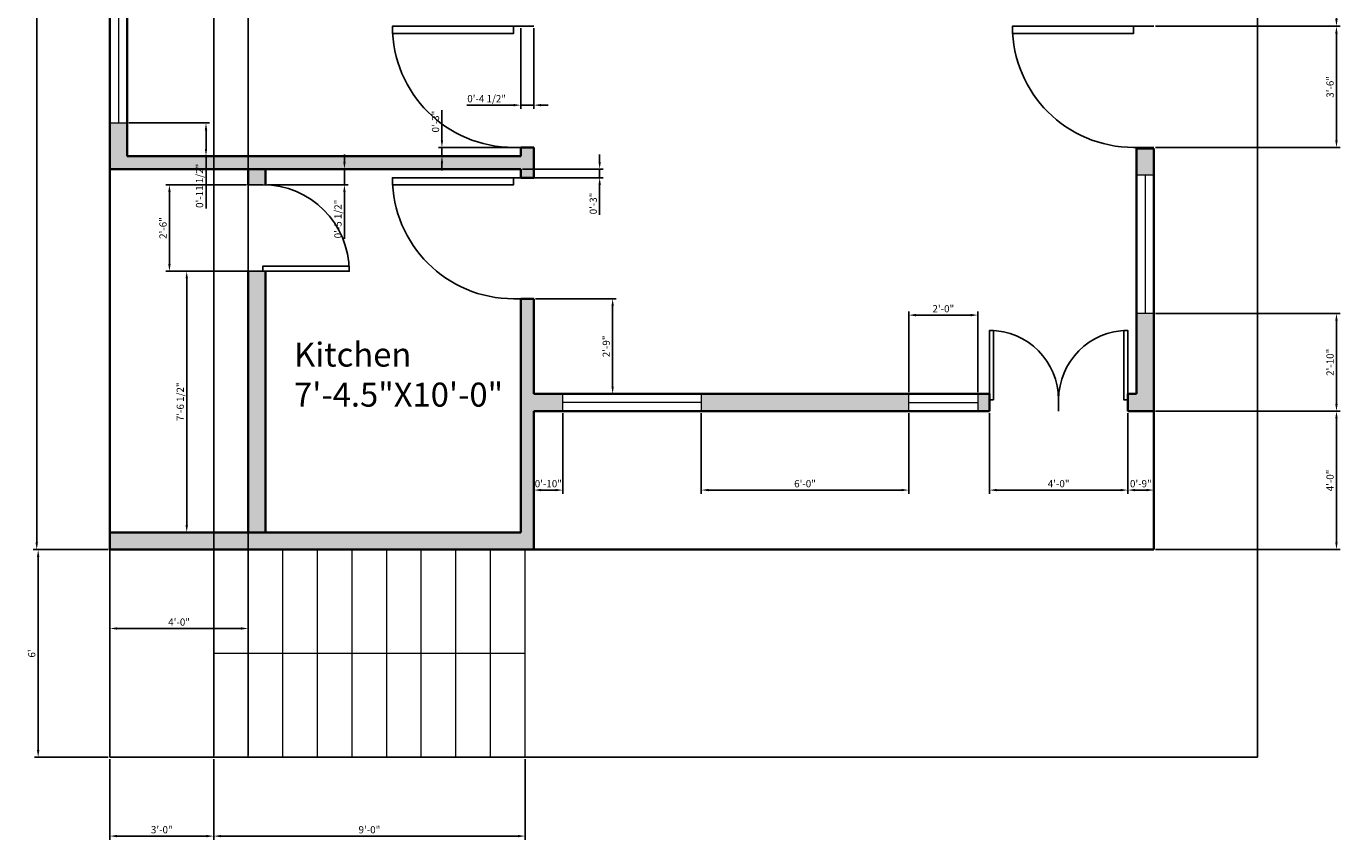
# Model space of a CAD drawing. Units: inches. Extents: x 1129603 to 1130059, y 1058961 to 1059552.
# Tile 1 of 2: x 1129603 to 1130059, y 1058961 to 1059243. Entities that reach past the tile are written whole.
import ezdxf

# ---------------------------------------------------------------- set-up
doc = ezdxf.new("R2010")
doc.units = ezdxf.units.IN
for name, color, linetype, lineweight in [('A-ANNO-DIMS', 2, 'Continuous', 18), ('A-AREA-IDEN', 7, 'Continuous', 25), ('A-DOOR', 3, 'Continuous', 25), ('A-FLOR-STRS', 7, 'Continuous', 18), ('A-GLAZ', 4, 'Continuous', 18), ('A-WALL-PATT', 9, 'Continuous', 13), ('C-PROP', 8, 'Continuous', 25), ('walls', 7, 'Continuous', 35)]:
    doc.layers.add(name, color=color, linetype=linetype, lineweight=lineweight)
doc.styles.get("Standard").update_dxf_attribs({"font": 'arial.ttf'})
doc.dimstyles.new('ISO-25', dxfattribs={"dimtxt": 2.5, "dimasz": 2.5, "dimexe": 1.25, "dimexo": 0.625, "dimtad": 1, "dimlunit": 4, "dimtxsty": 'Standard', "dimcen": 2.5, "dimadec": 0, "dimazin": 0, "dimtfac": 1, "dimtmove": 0, "dimatfit": 3, "dimfxl": 1, "dimarcsym": 0})

# ---------------------------------------------------------------- blocks, each defined once
blk = doc.blocks.new('*U2')
for p, q in [((0, 0), (0, -5)), ((30, 0), (30, -5))]:
    blk.add_line(p, q)
blk.add_lwpolyline([(0, 0), (0, 30), (1.75, 30), (1.75, 0)], close=True)
blk.add_arc((0, 0), 30, 0, 90)
blk = doc.blocks.new('*D5')
at = {"layer": 'A-ANNO-DIMS', "color": 0, "lineweight": -2, "transparency": 16777216}
for p, q in [((1129630.99, 1059520.87), (1129605, 1059520.87)), ((1129606.25, 1059518.37), (1129606.25, 1059064.37)), ((1129630.99, 1059061.87), (1129605, 1059061.87))]:
    blk.add_line(p, q, dxfattribs=at)
at = {"layer": 'A-ANNO-DIMS', "color": 0, "transparency": 16777216}
for points in [[(1129605.83, 1059518.37), (1129606.66, 1059518.37), (1129606.25, 1059520.87)], [(1129605.83, 1059064.37), (1129606.66, 1059064.37), (1129606.25, 1059061.87)]]:
    blk.add_solid(points, dxfattribs=at)
at = {"layer": 'Defpoints', "color": 0, "transparency": 16777216}
for p in [(1129631.62, 1059520.87), (1129606.25, 1059061.87), (1129631.62, 1059061.87)]:
    blk.add_point(p, dxfattribs=at)
at = {"layer": 'A-ANNO-DIMS', "color": 0, "transparency": 16777216, "insert": (1129604.34, 1059291.37), "char_height": 2.5, "attachment_point": 5, "rotation": 90}
blk.add_mtext('38\'-3"', dxfattribs=at)
blk = doc.blocks.new('*D6')
at = {"layer": 'A-ANNO-DIMS', "color": 0, "lineweight": -2, "transparency": 16777216}
for p, q in [((1129630.99, 1059061.87), (1129605.51, 1059061.87)), ((1129606.76, 1059059.37), (1129606.76, 1058992.37)), ((1129630.99, 1058989.87), (1129605.51, 1058989.87))]:
    blk.add_line(p, q, dxfattribs=at)
at = {"layer": 'A-ANNO-DIMS', "color": 0, "transparency": 16777216}
for points in [[(1129606.34, 1059059.37), (1129607.17, 1059059.37), (1129606.76, 1059061.87)], [(1129606.34, 1058992.37), (1129607.17, 1058992.37), (1129606.76, 1058989.87)]]:
    blk.add_solid(points, dxfattribs=at)
at = {"layer": 'Defpoints', "color": 0, "transparency": 16777216}
for p in [(1129631.62, 1059061.87), (1129606.76, 1058989.87), (1129631.62, 1058989.87)]:
    blk.add_point(p, dxfattribs=at)
at = {"layer": 'A-ANNO-DIMS', "color": 0, "transparency": 16777216, "insert": (1129604.85, 1059025.87), "char_height": 2.5, "attachment_point": 5, "rotation": 90}
blk.add_mtext("6'", dxfattribs=at)
blk = doc.blocks.new('WIN-48IN')
for p, q in [((0, 6), (48, 6)), ((0, 0), (0, 6)), ((48, 6), (48, 0)), ((0, 3), (48, 3)), ((48, 0), (0, 0))]:
    blk.add_line(p, q)
blk = doc.blocks.new('*D13')
at = {"layer": 'A-ANNO-DIMS', "color": 0, "lineweight": -2, "transparency": 16777216}
for p, q in [((1129638.24, 1059209.84), (1129666.21, 1059209.84)), ((1129664.96, 1059207.34), (1129664.96, 1059200.87)), ((1129638.24, 1059198.37), (1129666.21, 1059198.37)), ((1129664.96, 1059198.37), (1129664.96, 1059180.21))]:
    blk.add_line(p, q, dxfattribs=at)
at = {"layer": 'A-ANNO-DIMS', "color": 0, "transparency": 16777216}
for points in [[(1129664.54, 1059207.34), (1129665.37, 1059207.34), (1129664.96, 1059209.84)], [(1129664.54, 1059200.87), (1129665.37, 1059200.87), (1129664.96, 1059198.37)]]:
    blk.add_solid(points, dxfattribs=at)
at = {"layer": 'Defpoints', "color": 0, "transparency": 16777216}
for p in [(1129637.62, 1059209.84), (1129637.62, 1059198.37), (1129664.96, 1059198.37)]:
    blk.add_point(p, dxfattribs=at)
at = {"layer": 'A-ANNO-DIMS', "color": 0, "transparency": 16777216, "insert": (1129663.04, 1059188.04), "char_height": 2.5, "attachment_point": 5, "rotation": 90}
blk.add_mtext('0\'-11 1/2"', dxfattribs=at)
blk = doc.blocks.new('*D16')
at = {"layer": 'A-ANNO-DIMS', "color": 0, "lineweight": -2, "transparency": 16777216}
for p, q in [((1129994.24, 1059288.97), (1130058.21, 1059288.97)), ((1130056.96, 1059245.87), (1130056.96, 1059286.47)), ((1129994.24, 1059243.37), (1130058.21, 1059243.37))]:
    blk.add_line(p, q, dxfattribs=at)
at = {"layer": 'A-ANNO-DIMS', "color": 0, "transparency": 16777216}
for points in [[(1130056.54, 1059286.47), (1130057.37, 1059286.47), (1130056.96, 1059288.97)], [(1130056.54, 1059245.87), (1130057.37, 1059245.87), (1130056.96, 1059243.37)]]:
    blk.add_solid(points, dxfattribs=at)
at = {"layer": 'Defpoints', "color": 0, "transparency": 16777216}
for p in [(1129993.62, 1059288.97), (1130056.96, 1059288.97), (1129993.62, 1059243.37)]:
    blk.add_point(p, dxfattribs=at)
at = {"layer": 'A-ANNO-DIMS', "color": 0, "transparency": 16777216, "insert": (1130055.04, 1059266.17), "char_height": 2.5, "attachment_point": 5, "rotation": 90}
blk.add_mtext('3\'-9 1/2"', dxfattribs=at)
blk = doc.blocks.new('*D17')
at = {"layer": 'A-ANNO-DIMS', "color": 0, "lineweight": -2, "transparency": 16777216}
for p, q in [((1129994.24, 1059243.37), (1130058.21, 1059243.37)), ((1130056.96, 1059203.87), (1130056.96, 1059240.87)), ((1129994.24, 1059201.37), (1130058.21, 1059201.37))]:
    blk.add_line(p, q, dxfattribs=at)
at = {"layer": 'A-ANNO-DIMS', "color": 0, "transparency": 16777216}
for points in [[(1130056.54, 1059240.87), (1130057.37, 1059240.87), (1130056.96, 1059243.37)], [(1130056.54, 1059203.87), (1130057.37, 1059203.87), (1130056.96, 1059201.37)]]:
    blk.add_solid(points, dxfattribs=at)
at = {"layer": 'Defpoints', "color": 0, "transparency": 16777216}
for p in [(1129993.62, 1059243.37), (1130056.96, 1059243.37), (1129993.62, 1059201.37)]:
    blk.add_point(p, dxfattribs=at)
at = {"layer": 'A-ANNO-DIMS', "color": 0, "transparency": 16777216, "insert": (1130055.06, 1059222.37), "char_height": 2.5, "attachment_point": 5, "rotation": 90}
blk.add_mtext('3\'-6"', dxfattribs=at)
blk = doc.blocks.new('*D18')
at = {"layer": 'A-ANNO-DIMS', "color": 0, "lineweight": -2, "transparency": 16777216}
for p, q in [((1129994.24, 1059143.81), (1130058.21, 1059143.81)), ((1130056.96, 1059112.37), (1130056.96, 1059141.31)), ((1129994.24, 1059109.87), (1130058.21, 1059109.87))]:
    blk.add_line(p, q, dxfattribs=at)
at = {"layer": 'A-ANNO-DIMS', "color": 0, "transparency": 16777216}
for points in [[(1130056.54, 1059141.31), (1130057.37, 1059141.31), (1130056.96, 1059143.81)], [(1130056.54, 1059112.37), (1130057.37, 1059112.37), (1130056.96, 1059109.87)]]:
    blk.add_solid(points, dxfattribs=at)
at = {"layer": 'Defpoints', "color": 0, "transparency": 16777216}
for p in [(1129993.62, 1059143.81), (1130056.96, 1059143.81), (1129993.62, 1059109.87)]:
    blk.add_point(p, dxfattribs=at)
at = {"layer": 'A-ANNO-DIMS', "color": 0, "transparency": 16777216, "insert": (1130055.06, 1059126.84), "char_height": 2.5, "attachment_point": 5, "rotation": 90}
blk.add_mtext('2\'-10"', dxfattribs=at)
blk = doc.blocks.new('*D19')
at = {"layer": 'A-ANNO-DIMS', "color": 0, "lineweight": -2, "transparency": 16777216}
for p, q in [((1129994.24, 1059109.87), (1130058.21, 1059109.87)), ((1130056.96, 1059107.37), (1130056.96, 1059064.37)), ((1129994.24, 1059061.87), (1130058.21, 1059061.87))]:
    blk.add_line(p, q, dxfattribs=at)
at = {"layer": 'A-ANNO-DIMS', "color": 0, "transparency": 16777216}
for points in [[(1130056.54, 1059107.37), (1130057.37, 1059107.37), (1130056.96, 1059109.87)], [(1130056.54, 1059064.37), (1130057.37, 1059064.37), (1130056.96, 1059061.87)]]:
    blk.add_solid(points, dxfattribs=at)
at = {"layer": 'Defpoints', "color": 0, "transparency": 16777216}
for p in [(1129993.62, 1059109.87), (1129993.62, 1059061.87), (1130056.96, 1059061.87)]:
    blk.add_point(p, dxfattribs=at)
at = {"layer": 'A-ANNO-DIMS', "color": 0, "transparency": 16777216, "insert": (1130055.06, 1059085.87), "char_height": 2.5, "attachment_point": 5, "rotation": 90}
blk.add_mtext('4\'-0"', dxfattribs=at)
blk = doc.blocks.new('*D20')
at = {"layer": 'A-ANNO-DIMS', "color": 0, "lineweight": -2, "transparency": 16777216}
for p, q in [((1129631.62, 1059061.25), (1129631.62, 1059033.28)), ((1129679.62, 1059061.25), (1129679.62, 1059033.28)), ((1129677.12, 1059034.53), (1129634.12, 1059034.53))]:
    blk.add_line(p, q, dxfattribs=at)
at = {"layer": 'A-ANNO-DIMS', "color": 0, "transparency": 16777216}
for points in [[(1129634.12, 1059034.95), (1129634.12, 1059034.12), (1129631.62, 1059034.53)], [(1129677.12, 1059034.95), (1129677.12, 1059034.12), (1129679.62, 1059034.53)]]:
    blk.add_solid(points, dxfattribs=at)
at = {"layer": 'Defpoints', "color": 0, "transparency": 16777216}
for p in [(1129631.62, 1059061.87), (1129679.62, 1059061.87), (1129631.62, 1059034.53)]:
    blk.add_point(p, dxfattribs=at)
at = {"layer": 'A-ANNO-DIMS', "color": 0, "transparency": 16777216, "insert": (1129655.62, 1059036.43), "char_height": 2.5, "attachment_point": 5}
blk.add_mtext('4\'-0"', dxfattribs=at)
blk = doc.blocks.new('*D21')
at = {"layer": 'A-ANNO-DIMS', "color": 0, "lineweight": -2, "transparency": 16777216}
for p, q in [((1129631.62, 1058989.25), (1129631.62, 1058961.28)), ((1129667.62, 1058989.25), (1129667.62, 1058961.28)), ((1129634.12, 1058962.53), (1129665.12, 1058962.53))]:
    blk.add_line(p, q, dxfattribs=at)
at = {"layer": 'A-ANNO-DIMS', "color": 0, "transparency": 16777216}
for points in [[(1129634.12, 1058962.95), (1129634.12, 1058962.12), (1129631.62, 1058962.53)], [(1129665.12, 1058962.95), (1129665.12, 1058962.12), (1129667.62, 1058962.53)]]:
    blk.add_solid(points, dxfattribs=at)
at = {"layer": 'Defpoints', "color": 0, "transparency": 16777216}
for p in [(1129631.62, 1058989.87), (1129667.62, 1058989.87), (1129667.62, 1058962.53)]:
    blk.add_point(p, dxfattribs=at)
at = {"layer": 'A-ANNO-DIMS', "color": 0, "transparency": 16777216, "insert": (1129649.62, 1058964.43), "char_height": 2.5, "attachment_point": 5}
blk.add_mtext('3\'-0"', dxfattribs=at)
blk = doc.blocks.new('*D22')
at = {"layer": 'A-ANNO-DIMS', "color": 0, "lineweight": -2, "transparency": 16777216}
for p, q in [((1129667.62, 1058989.25), (1129667.62, 1058961.28)), ((1129775.62, 1058989.25), (1129775.62, 1058961.28)), ((1129670.12, 1058962.53), (1129773.12, 1058962.53))]:
    blk.add_line(p, q, dxfattribs=at)
at = {"layer": 'A-ANNO-DIMS', "color": 0, "transparency": 16777216}
for points in [[(1129670.12, 1058962.95), (1129670.12, 1058962.12), (1129667.62, 1058962.53)], [(1129773.12, 1058962.95), (1129773.12, 1058962.12), (1129775.62, 1058962.53)]]:
    blk.add_solid(points, dxfattribs=at)
at = {"layer": 'Defpoints', "color": 0, "transparency": 16777216}
for p in [(1129667.62, 1058989.87), (1129775.62, 1058989.87), (1129775.62, 1058962.53)]:
    blk.add_point(p, dxfattribs=at)
at = {"layer": 'A-ANNO-DIMS', "color": 0, "transparency": 16777216, "insert": (1129721.62, 1058964.43), "char_height": 2.5, "attachment_point": 5}
blk.add_mtext('9\'-0"', dxfattribs=at)
blk = doc.blocks.new('*D23')
at = {"layer": 'A-ANNO-DIMS', "color": 0, "lineweight": -2, "transparency": 16777216}
for p, q in [((1129667.62, 1058990.5), (1129667.62, 1059549.47)), ((1129670.12, 1059548.22), (1129677.12, 1059548.22)), ((1129679.62, 1058990.5), (1129679.62, 1059549.47))]:
    blk.add_line(p, q, dxfattribs=at)
at = {"layer": 'A-ANNO-DIMS', "color": 0, "transparency": 16777216}
for points in [[(1129670.12, 1059548.63), (1129670.12, 1059547.8), (1129667.62, 1059548.22)], [(1129677.12, 1059548.63), (1129677.12, 1059547.8), (1129679.62, 1059548.22)]]:
    blk.add_solid(points, dxfattribs=at)
at = {"layer": 'Defpoints', "color": 0, "transparency": 16777216}
for p in [(1129679.62, 1059548.22), (1129667.62, 1058989.87), (1129679.62, 1058989.87)]:
    blk.add_point(p, dxfattribs=at)
at = {"layer": 'A-ANNO-DIMS', "color": 0, "transparency": 16777216, "insert": (1129673.62, 1059550.12), "char_height": 2.5, "attachment_point": 5}
blk.add_mtext('1\'-0"', dxfattribs=at)
blk = doc.blocks.new('*D24')
at = {"layer": 'A-ANNO-DIMS', "color": 0, "lineweight": -2, "transparency": 16777216}
for p, q in [((1129936.62, 1059109.25), (1129936.62, 1059081.28)), ((1129984.62, 1059109.25), (1129984.62, 1059081.28)), ((1129982.12, 1059082.53), (1129939.12, 1059082.53))]:
    blk.add_line(p, q, dxfattribs=at)
at = {"layer": 'A-ANNO-DIMS', "color": 0, "transparency": 16777216}
for points in [[(1129939.12, 1059082.95), (1129939.12, 1059082.12), (1129936.62, 1059082.53)], [(1129982.12, 1059082.95), (1129982.12, 1059082.12), (1129984.62, 1059082.53)]]:
    blk.add_solid(points, dxfattribs=at)
at = {"layer": 'Defpoints', "color": 0, "transparency": 16777216}
for p in [(1129936.62, 1059109.87), (1129984.62, 1059109.87), (1129936.62, 1059082.53)]:
    blk.add_point(p, dxfattribs=at)
at = {"layer": 'A-ANNO-DIMS', "color": 0, "transparency": 16777216, "insert": (1129960.62, 1059084.43), "char_height": 2.5, "attachment_point": 5, "rotation": 0}
blk.add_mtext('4\'-0"', dxfattribs=at)
blk = doc.blocks.new('*D25')
at = {"layer": 'A-ANNO-DIMS', "color": 0, "lineweight": -2, "transparency": 16777216}
for p, q in [((1129908.63, 1059116.5), (1129908.63, 1059144.47)), ((1129932.63, 1059116.5), (1129932.63, 1059144.47)), ((1129911.13, 1059143.22), (1129930.13, 1059143.22))]:
    blk.add_line(p, q, dxfattribs=at)
at = {"layer": 'A-ANNO-DIMS', "color": 0, "transparency": 16777216}
for points in [[(1129911.13, 1059143.63), (1129911.13, 1059142.8), (1129908.63, 1059143.22)], [(1129930.13, 1059143.63), (1129930.13, 1059142.8), (1129932.63, 1059143.22)]]:
    blk.add_solid(points, dxfattribs=at)
at = {"layer": 'Defpoints', "color": 0, "transparency": 16777216}
for p in [(1129932.63, 1059143.22), (1129908.63, 1059115.87), (1129932.63, 1059115.87)]:
    blk.add_point(p, dxfattribs=at)
at = {"layer": 'A-ANNO-DIMS', "color": 0, "transparency": 16777216, "insert": (1129920.63, 1059145.12), "char_height": 2.5, "attachment_point": 5}
blk.add_mtext('2\'-0"', dxfattribs=at)
blk = doc.blocks.new('*D26')
at = {"layer": 'A-ANNO-DIMS', "color": 0, "lineweight": -2, "transparency": 16777216}
for p, q in [((1129778.62, 1059109.25), (1129778.62, 1059081.28)), ((1129788.71, 1059109.25), (1129788.71, 1059081.28)), ((1129786.21, 1059082.53), (1129781.12, 1059082.53))]:
    blk.add_line(p, q, dxfattribs=at)
at = {"layer": 'A-ANNO-DIMS', "color": 0, "transparency": 16777216}
for points in [[(1129781.12, 1059082.95), (1129781.12, 1059082.12), (1129778.62, 1059082.53)], [(1129786.21, 1059082.95), (1129786.21, 1059082.12), (1129788.71, 1059082.53)]]:
    blk.add_solid(points, dxfattribs=at)
at = {"layer": 'Defpoints', "color": 0, "transparency": 16777216}
for p in [(1129778.62, 1059109.87), (1129788.71, 1059109.87), (1129778.62, 1059082.53)]:
    blk.add_point(p, dxfattribs=at)
at = {"layer": 'A-ANNO-DIMS', "color": 0, "transparency": 16777216, "insert": (1129783.66, 1059084.43), "char_height": 2.5, "attachment_point": 5, "rotation": 0}
blk.add_mtext('0\'-10"', dxfattribs=at)
blk = doc.blocks.new('*D27')
at = {"layer": 'A-ANNO-DIMS', "color": 0, "lineweight": -2, "transparency": 16777216}
for p, q in [((1129836.71, 1059109.25), (1129836.71, 1059081.28)), ((1129908.63, 1059109.25), (1129908.63, 1059081.28)), ((1129906.13, 1059082.53), (1129839.21, 1059082.53))]:
    blk.add_line(p, q, dxfattribs=at)
at = {"layer": 'A-ANNO-DIMS', "color": 0, "transparency": 16777216}
for points in [[(1129839.21, 1059082.95), (1129839.21, 1059082.12), (1129836.71, 1059082.53)], [(1129906.13, 1059082.95), (1129906.13, 1059082.12), (1129908.63, 1059082.53)]]:
    blk.add_solid(points, dxfattribs=at)
at = {"layer": 'Defpoints', "color": 0, "transparency": 16777216}
for p in [(1129836.71, 1059109.87), (1129908.63, 1059109.87), (1129836.71, 1059082.53)]:
    blk.add_point(p, dxfattribs=at)
at = {"layer": 'A-ANNO-DIMS', "color": 0, "transparency": 16777216, "insert": (1129872.67, 1059084.43), "char_height": 2.5, "attachment_point": 5, "rotation": 0}
blk.add_mtext('6\'-0"', dxfattribs=at)
blk = doc.blocks.new('*D28')
at = {"layer": 'A-ANNO-DIMS', "color": 0, "lineweight": -2, "transparency": 16777216}
for p, q in [((1129984.62, 1059109.25), (1129984.62, 1059081.28)), ((1129993.62, 1059109.25), (1129993.62, 1059081.28)), ((1129991.12, 1059082.53), (1129987.12, 1059082.53))]:
    blk.add_line(p, q, dxfattribs=at)
at = {"layer": 'A-ANNO-DIMS', "color": 0, "transparency": 16777216}
for points in [[(1129987.12, 1059082.95), (1129987.12, 1059082.12), (1129984.62, 1059082.53)], [(1129991.12, 1059082.95), (1129991.12, 1059082.12), (1129993.62, 1059082.53)]]:
    blk.add_solid(points, dxfattribs=at)
at = {"layer": 'Defpoints', "color": 0, "transparency": 16777216}
for p in [(1129984.62, 1059109.87), (1129993.62, 1059109.87), (1129984.62, 1059082.53)]:
    blk.add_point(p, dxfattribs=at)
at = {"layer": 'A-ANNO-DIMS', "color": 0, "transparency": 16777216, "insert": (1129989.12, 1059084.43), "char_height": 2.5, "attachment_point": 5}
blk.add_mtext('0\'-9"', dxfattribs=at)
blk = doc.blocks.new('*D36')
at = {"layer": 'A-ANNO-DIMS', "color": 0, "lineweight": -2, "transparency": 16777216}
for p, q in [((1129678.99, 1059188.42), (1129651.02, 1059188.42)), ((1129652.27, 1059160.92), (1129652.27, 1059185.92)), ((1129678.99, 1059158.42), (1129651.02, 1059158.42))]:
    blk.add_line(p, q, dxfattribs=at)
at = {"layer": 'A-ANNO-DIMS', "color": 0, "transparency": 16777216}
for points in [[(1129651.86, 1059185.92), (1129652.69, 1059185.92), (1129652.27, 1059188.42)], [(1129651.86, 1059160.92), (1129652.69, 1059160.92), (1129652.27, 1059158.42)]]:
    blk.add_solid(points, dxfattribs=at)
at = {"layer": 'Defpoints', "color": 0, "transparency": 16777216}
for p in [(1129652.27, 1059188.42), (1129679.62, 1059188.42), (1129679.62, 1059158.42)]:
    blk.add_point(p, dxfattribs=at)
at = {"layer": 'A-ANNO-DIMS', "color": 0, "transparency": 16777216, "insert": (1129650.37, 1059173.42), "char_height": 2.5, "attachment_point": 5, "rotation": 90}
blk.add_mtext('2\'-6"', dxfattribs=at)
blk = doc.blocks.new('*D37')
at = {"layer": 'A-ANNO-DIMS', "color": 0, "lineweight": -2, "transparency": 16777216}
for p, q in [((1129801.46, 1059196.37), (1129801.46, 1059198.87)), ((1129774.74, 1059193.87), (1129802.71, 1059193.87)), ((1129774.74, 1059190.87), (1129802.71, 1059190.87)), ((1129801.46, 1059193.87), (1129801.46, 1059190.87)), ((1129801.46, 1059188.37), (1129801.46, 1059177.98))]:
    blk.add_line(p, q, dxfattribs=at)
at = {"layer": 'A-ANNO-DIMS', "color": 0, "transparency": 16777216}
for points in [[(1129801.04, 1059196.37), (1129801.87, 1059196.37), (1129801.46, 1059193.87)], [(1129801.04, 1059188.37), (1129801.87, 1059188.37), (1129801.46, 1059190.87)]]:
    blk.add_solid(points, dxfattribs=at)
at = {"layer": 'Defpoints', "color": 0, "transparency": 16777216}
for p in [(1129774.12, 1059193.87), (1129774.12, 1059190.87), (1129801.46, 1059190.87)]:
    blk.add_point(p, dxfattribs=at)
at = {"layer": 'A-ANNO-DIMS', "color": 0, "transparency": 16777216, "insert": (1129799.56, 1059181.93), "char_height": 2.5, "attachment_point": 5, "rotation": 90}
blk.add_mtext('0\'-3"', dxfattribs=at)
blk = doc.blocks.new('*D38')
at = {"layer": 'A-ANNO-DIMS', "color": 0, "lineweight": -2, "transparency": 16777216}
for p, q in [((1129746.77, 1059203.87), (1129746.77, 1059214.27)), ((1129773.49, 1059201.37), (1129745.52, 1059201.37)), ((1129746.77, 1059198.37), (1129746.77, 1059201.37)), ((1129773.49, 1059198.37), (1129745.52, 1059198.37)), ((1129746.77, 1059195.87), (1129746.77, 1059193.37))]:
    blk.add_line(p, q, dxfattribs=at)
at = {"layer": 'A-ANNO-DIMS', "color": 0, "transparency": 16777216}
for points in [[(1129746.36, 1059203.87), (1129747.19, 1059203.87), (1129746.77, 1059201.37)], [(1129746.36, 1059195.87), (1129747.19, 1059195.87), (1129746.77, 1059198.37)]]:
    blk.add_solid(points, dxfattribs=at)
at = {"layer": 'Defpoints', "color": 0, "transparency": 16777216}
for p in [(1129746.77, 1059201.37), (1129774.12, 1059201.37), (1129774.12, 1059198.37)]:
    blk.add_point(p, dxfattribs=at)
at = {"layer": 'A-ANNO-DIMS', "color": 0, "transparency": 16777216, "insert": (1129744.87, 1059210.32), "char_height": 2.5, "attachment_point": 5, "rotation": 90}
blk.add_mtext('0\'-3"', dxfattribs=at)
blk = doc.blocks.new('*D40')
at = {"layer": 'A-ANNO-DIMS', "color": 0, "lineweight": -2, "transparency": 16777216}
for p, q in [((1129774.12, 1059242.75), (1129774.12, 1059214.78)), ((1129778.62, 1059242.75), (1129778.62, 1059214.78)), ((1129771.62, 1059216.03), (1129755.39, 1059216.03)), ((1129778.62, 1059216.03), (1129774.12, 1059216.03)), ((1129781.12, 1059216.03), (1129783.62, 1059216.03))]:
    blk.add_line(p, q, dxfattribs=at)
at = {"layer": 'A-ANNO-DIMS', "color": 0, "transparency": 16777216}
for points in [[(1129771.62, 1059216.45), (1129771.62, 1059215.62), (1129774.12, 1059216.03)], [(1129781.12, 1059216.45), (1129781.12, 1059215.62), (1129778.62, 1059216.03)]]:
    blk.add_solid(points, dxfattribs=at)
at = {"layer": 'Defpoints', "color": 0, "transparency": 16777216}
for p in [(1129774.12, 1059243.37), (1129778.62, 1059243.37), (1129774.12, 1059216.03)]:
    blk.add_point(p, dxfattribs=at)
at = {"layer": 'A-ANNO-DIMS', "color": 0, "transparency": 16777216, "insert": (1129762.26, 1059217.95), "char_height": 2.5, "attachment_point": 5}
blk.add_mtext('0\'-4 1/2"', dxfattribs=at)
blk = doc.blocks.new('*D41')
at = {"layer": 'A-ANNO-DIMS', "color": 0, "lineweight": -2, "transparency": 16777216}
for p, q in [((1129712.96, 1059196.37), (1129712.96, 1059198.87)), ((1129686.24, 1059193.87), (1129714.21, 1059193.87)), ((1129712.96, 1059193.87), (1129712.96, 1059188.4)), ((1129686.24, 1059188.4), (1129714.21, 1059188.4)), ((1129712.96, 1059185.9), (1129712.96, 1059169.68))]:
    blk.add_line(p, q, dxfattribs=at)
at = {"layer": 'A-ANNO-DIMS', "color": 0, "transparency": 16777216}
for points in [[(1129712.54, 1059196.37), (1129713.37, 1059196.37), (1129712.96, 1059193.87)], [(1129712.54, 1059185.9), (1129713.37, 1059185.9), (1129712.96, 1059188.4)]]:
    blk.add_solid(points, dxfattribs=at)
at = {"layer": 'Defpoints', "color": 0, "transparency": 16777216}
for p in [(1129685.62, 1059193.87), (1129685.62, 1059188.4), (1129712.96, 1059188.4)]:
    blk.add_point(p, dxfattribs=at)
at = {"layer": 'A-ANNO-DIMS', "color": 0, "transparency": 16777216, "insert": (1129711.04, 1059176.54), "char_height": 2.5, "attachment_point": 5, "rotation": 90}
blk.add_mtext('0\'-5 1/2"', dxfattribs=at)
blk = doc.blocks.new('*D42')
at = {"layer": 'A-ANNO-DIMS', "color": 0, "lineweight": -2, "transparency": 16777216}
for p, q in [((1129684.99, 1059158.42), (1129657.02, 1059158.42)), ((1129658.27, 1059070.37), (1129658.27, 1059155.92)), ((1129684.99, 1059067.87), (1129657.02, 1059067.87))]:
    blk.add_line(p, q, dxfattribs=at)
at = {"layer": 'A-ANNO-DIMS', "color": 0, "transparency": 16777216}
for points in [[(1129657.86, 1059155.92), (1129658.69, 1059155.92), (1129658.27, 1059158.42)], [(1129657.86, 1059070.37), (1129658.69, 1059070.37), (1129658.27, 1059067.87)]]:
    blk.add_solid(points, dxfattribs=at)
at = {"layer": 'Defpoints', "color": 0, "transparency": 16777216}
for p in [(1129658.27, 1059158.42), (1129685.62, 1059158.42), (1129685.62, 1059067.87)]:
    blk.add_point(p, dxfattribs=at)
at = {"layer": 'A-ANNO-DIMS', "color": 0, "transparency": 16777216, "insert": (1129656.36, 1059113.15), "char_height": 2.5, "attachment_point": 5, "rotation": 90}
blk.add_mtext('7\'-6 1/2"', dxfattribs=at)
blk = doc.blocks.new('*D44')
at = {"layer": 'A-ANNO-DIMS', "color": 0, "lineweight": -2, "transparency": 16777216}
for p, q in [((1129779.24, 1059148.87), (1129807.21, 1059148.87)), ((1129805.96, 1059146.37), (1129805.96, 1059118.37)), ((1129779.24, 1059115.87), (1129807.21, 1059115.87))]:
    blk.add_line(p, q, dxfattribs=at)
at = {"layer": 'A-ANNO-DIMS', "color": 0, "transparency": 16777216}
for points in [[(1129805.54, 1059146.37), (1129806.37, 1059146.37), (1129805.96, 1059148.87)], [(1129805.54, 1059118.37), (1129806.37, 1059118.37), (1129805.96, 1059115.87)]]:
    blk.add_solid(points, dxfattribs=at)
at = {"layer": 'Defpoints', "color": 0, "transparency": 16777216}
for p in [(1129778.62, 1059148.87), (1129778.62, 1059115.87), (1129805.96, 1059115.87)]:
    blk.add_point(p, dxfattribs=at)
at = {"layer": 'A-ANNO-DIMS', "color": 0, "transparency": 16777216, "insert": (1129804.06, 1059132.37), "char_height": 2.5, "attachment_point": 5, "rotation": 90}
blk.add_mtext('2\'-9"', dxfattribs=at)

msp = doc.modelspace()

# ---------------------------------------------------------------- hatches: boundary and pattern name
at = {"layer": 'A-WALL-PATT'}
h = msp.add_hatch(color=256, dxfattribs=at)
h.dxf.hatch_style = 1
h.paths.add_polyline_path([(1129778.616, 1059201.374), (1129774.116, 1059201.374), (1129774.116, 1059198.374), (1129637.616, 1059198.374), (1129637.616, 1059209.837), (1129631.616, 1059209.837), (1129631.616, 1059193.874), (1129774.116, 1059193.874), (1129774.116, 1059190.874), (1129778.616, 1059190.874)])
h = msp.add_hatch(color=256, dxfattribs=at)
h.dxf.hatch_style = 1
h.paths.add_polyline_path([(1129993.616, 1059200.948), (1129987.616, 1059200.948), (1129987.616, 1059191.808), (1129993.616, 1059191.808)])
h = msp.add_hatch(color=256, dxfattribs=at)
h.dxf.hatch_style = 1
h.paths.add_polyline_path([(1129685.616, 1059193.874), (1129679.616, 1059193.874), (1129679.616, 1059188.416), (1129684.616, 1059188.416, -0.0083351), (1129685.616, 1059188.399)])
h = msp.add_hatch(color=256, dxfattribs=at)
h.dxf.hatch_style = 1
h.paths.add_polyline_path([(1129685.616, 1059158.416), (1129684.616, 1059158.416), (1129679.616, 1059158.416), (1129679.616, 1059067.874), (1129685.616, 1059067.874)])
h = msp.add_hatch(color=256, dxfattribs=at)
h.dxf.hatch_style = 1
h.paths.add_polyline_path([(1129788.714, 1059115.874), (1129778.616, 1059115.874), (1129778.616, 1059148.874), (1129774.116, 1059148.874), (1129774.116, 1059067.874), (1129631.616, 1059067.874), (1129631.616, 1059061.874), (1129778.616, 1059061.874), (1129778.616, 1059109.874), (1129788.714, 1059109.874)])
h = msp.add_hatch(color=256, dxfattribs=at)
h.dxf.hatch_style = 1
h.paths.add_polyline_path([(1129993.616, 1059143.808), (1129987.616, 1059143.808), (1129987.616, 1059115.874), (1129984.616, 1059115.874), (1129984.616, 1059113.874), (1129984.616, 1059109.874), (1129993.616, 1059109.874)])
h = msp.add_hatch(color=256, dxfattribs=at)
h.dxf.hatch_style = 1
h.paths.add_polyline_path([(1129908.631, 1059115.874), (1129836.714, 1059115.874), (1129836.714, 1059109.874), (1129908.631, 1059109.874)])
h = msp.add_hatch(color=256, dxfattribs=at)
h.dxf.hatch_style = 1
h.paths.add_polyline_path([(1129936.616, 1059115.874), (1129932.631, 1059115.874), (1129932.631, 1059109.874), (1129936.616, 1059109.874), (1129936.616, 1059113.874)])

# ---------------------------------------------------------------- linework, layer by layer
at = {"layer": 'A-FLOR-STRS'}
for p, q in [((1129667.616, 1058989.874), (1129667.616, 1059061.874)), ((1129679.616, 1058989.874), (1129679.616, 1059061.874)), ((1129691.616, 1058989.874), (1129691.616, 1059061.874)), ((1129703.616, 1058989.874), (1129703.616, 1059061.874)), ((1129715.616, 1058989.874), (1129715.616, 1059061.874)), ((1129727.616, 1058989.874), (1129727.616, 1059061.874)), ((1129739.616, 1058989.874), (1129739.616, 1059061.874)), ((1129751.616, 1058989.874), (1129751.616, 1059061.874)), ((1129763.616, 1058989.874), (1129763.616, 1059061.874)), ((1129775.616, 1058989.874), (1129775.616, 1059061.874)), ((1129775.616, 1059025.874), (1129667.616, 1059025.874))]:
    msp.add_line(p, q, dxfattribs=at)
at = {"layer": 'A-GLAZ'}
for p, q in [((1129908.631, 1059115.874), (1129932.631, 1059115.874)), ((1129908.631, 1059109.874), (1129908.631, 1059115.874)), ((1129908.631, 1059112.874), (1129932.631, 1059112.874)), ((1129932.631, 1059115.874), (1129932.631, 1059109.874)), ((1129932.631, 1059109.874), (1129908.631, 1059109.874))]:
    msp.add_line(p, q, dxfattribs=at)
at = {"layer": 'C-PROP'}
for p, q in [((1130029.616, 1059520.874), (1130029.616, 1059061.874)), ((1129631.616, 1058989.874), (1129631.616, 1059061.874)), ((1130029.616, 1059061.874), (1130029.616, 1058989.874)), ((1130029.616, 1058989.874), (1129631.616, 1058989.874))]:
    msp.add_line(p, q, dxfattribs=at)
at = {"layer": 'walls'}
for p, q in [((1129631.616, 1059061.874), (1129631.616, 1059520.874)), ((1129637.616, 1059198.374), (1129637.616, 1059318.374)), ((1129774.116, 1059198.374), (1129774.116, 1059201.374)), ((1129774.116, 1059198.374), (1129774.116, 1059201.374)), ((1129774.116, 1059201.374), (1129778.616, 1059201.374)), ((1129778.616, 1059190.874), (1129778.616, 1059201.374)), ((1129987.616, 1059200.948), (1129993.616, 1059200.948)), ((1129987.616, 1059200.948), (1129987.616, 1059115.874)), ((1129993.616, 1059200.948), (1129993.616, 1059109.874)), ((1129637.616, 1059198.374), (1129774.116, 1059198.374)), ((1129631.616, 1059193.874), (1129774.116, 1059193.874)), ((1129679.616, 1059188.416), (1129679.616, 1059193.874)), ((1129685.616, 1059188.399), (1129685.616, 1059193.874)), ((1129774.116, 1059193.874), (1129774.116, 1059190.874)), ((1129774.116, 1059190.874), (1129774.116, 1059193.874)), ((1129774.116, 1059190.874), (1129778.616, 1059190.874)), ((1129679.616, 1059067.874), (1129679.616, 1059158.416)), ((1129685.616, 1059067.874), (1129685.616, 1059158.416)), ((1129774.116, 1059067.874), (1129774.116, 1059148.874)), ((1129778.616, 1059148.874), (1129774.116, 1059148.874)), ((1129778.616, 1059115.874), (1129778.616, 1059148.874)), ((1129936.616, 1059115.874), (1129778.616, 1059115.874)), ((1129936.616, 1059109.874), (1129936.616, 1059115.874)), ((1129987.616, 1059115.874), (1129984.616, 1059115.874)), ((1129987.616, 1059115.874), (1129984.616, 1059115.874)), ((1129984.616, 1059115.874), (1129984.616, 1059109.874)), ((1129778.616, 1059061.874), (1129778.616, 1059109.874)), ((1129936.616, 1059109.874), (1129778.616, 1059109.874)), ((1129993.616, 1059109.874), (1129984.616, 1059109.874)), ((1129993.616, 1059109.874), (1129993.616, 1059061.874)), ((1129774.116, 1059067.874), (1129631.616, 1059067.874)), ((1129993.616, 1059061.874), (1129631.616, 1059061.874))]:
    msp.add_line(p, q, dxfattribs=at)

# ---------------------------------------------------------------- block references
at = {"layer": 'A-DOOR', "xscale": -1.399999999999999, "yscale": 1.399999999999999, "zscale": 1.399999999999999, "rotation": 90}
for p in [(1129771.616, 1059243.374), (1129986.616, 1059243.374), (1129771.616, 1059190.874)]:
    msp.add_blockref('*U2', p, dxfattribs=at)
at = {"layer": 'A-DOOR', "xscale": -1, "rotation": 270}
msp.add_blockref('*U2', (1129684.616, 1059158.416), dxfattribs=at)
at = {"layer": 'A-DOOR', "yscale": 0.8, "zscale": 0.8}
for p, xscale in [((1129936.616, 1059113.874), 0.8), ((1129984.616, 1059113.874), -0.8)]:
    msp.add_blockref('*U2', p, dxfattribs=dict(at, xscale=xscale))
at = {"layer": 'A-GLAZ'}
for p, rotation in [((1129631.616, 1059257.837), 269.9999999996579), ((1129987.616, 1059191.808), 270.0000000002053), ((1129836.714, 1059115.874), 180)]:
    msp.add_blockref('WIN-48IN', p, dxfattribs=dict(at, rotation=rotation))

# ---------------------------------------------------------------- texts
at = {"layer": 'A-AREA-IDEN', "insert": (1129695.476, 1059133.692), "char_height": 8.33239, "attachment_point": 1}
msp.add_mtext_dynamic_manual_height_columns('Kitchen\\P7\'-4.5"X10\'-0"', width=13.35039, gutter_width=41.662, heights=[0], dxfattribs=at)

# ---------------------------------------------------------------- dimensions: what is measured, and where the dimension line sits
at = {"layer": 'A-ANNO-DIMS'}
for base, p1, p2, picture, middle in [((1129679.616, 1059548.217), (1129667.616, 1058989.874), (1129679.616, 1058989.874), '*D23', (1129673.616, 1059550.118)), ((1129932.631, 1059143.217), (1129908.631, 1059115.874), (1129932.631, 1059115.874), '*D25', (1129920.631, 1059145.118)), ((1129667.616, 1058962.532), (1129631.616, 1058989.874), (1129667.616, 1058989.874), '*D21', (1129649.616, 1058964.434)), ((1129775.616, 1058962.532), (1129667.616, 1058989.874), (1129775.616, 1058989.874), '*D22', (1129721.616, 1058964.433))]:
    dim = msp.add_linear_dim(base=base, p1=p1, p2=p2, dimstyle='ISO-25', override={"dimdec": 1, "dimlfac": 1, "dimrnd": 0, "dimzin": 1, "dimdsep": 46, "dimlunit": 4, "dimfrac": 2}, dxfattribs=at)
    dim.commit()
    dim.dimension.update_dxf_attribs({"geometry": picture, "text_midpoint": middle})
for base, p1, p2, angle, override, picture, middle in [((1129606.247, 1059061.874), (1129631.616, 1059520.874), (1129631.616, 1059061.874), 90, {"dimclrd": 0, "dimclre": 0, "dimclrt": 0}, '*D5', (1129604.345, 1059291.374)), ((1130056.958, 1059288.967), (1129993.616, 1059243.374), (1129993.616, 1059288.967), 90, {"dimdec": 1, "dimlfac": 1, "dimrnd": 0, "dimzin": 1, "dimdsep": 46, "dimlunit": 4, "dimfrac": 2}, '*D16', (1130055.04, 1059266.171)), ((1129774.116, 1059216.032), (1129778.616, 1059243.374), (1129774.116, 1059243.374), 180, {"dimdec": 1, "dimlfac": 1, "dimrnd": 0, "dimzin": 1, "dimdsep": 46, "dimlunit": 4, "dimfrac": 2}, '*D40', (1129762.255, 1059217.949)), ((1130056.958, 1059243.374), (1129993.616, 1059201.374), (1129993.616, 1059243.374), 90, {"dimdec": 1, "dimlfac": 1, "dimrnd": 0, "dimzin": 1, "dimdsep": 46, "dimlunit": 4, "dimfrac": 2}, '*D17', (1130055.056, 1059222.374)), ((1129746.773, 1059201.374), (1129774.116, 1059198.374), (1129774.116, 1059201.374), 90, {"dimdec": 1, "dimlfac": 1, "dimrnd": 0, "dimzin": 1, "dimdsep": 46, "dimlunit": 4, "dimfrac": 2}, '*D38', (1129744.871, 1059210.322)), ((1129664.958, 1059198.374), (1129637.616, 1059209.837), (1129637.616, 1059198.374), 270, {"dimdec": 1, "dimlfac": 1, "dimrnd": 0, "dimzin": 1, "dimdsep": 46, "dimlunit": 4, "dimfrac": 2}, '*D13', (1129663.041, 1059188.043)), ((1129712.958, 1059188.399), (1129685.616, 1059193.874), (1129685.616, 1059188.399), 270, {"dimdec": 1, "dimlfac": 1, "dimrnd": 0, "dimzin": 1, "dimdsep": 46, "dimlunit": 4, "dimfrac": 2}, '*D41', (1129711.041, 1059176.539)), ((1129801.458, 1059190.874), (1129774.116, 1059193.874), (1129774.116, 1059190.874), 270, {"dimdec": 1, "dimlfac": 1, "dimrnd": 0, "dimzin": 1, "dimdsep": 46, "dimlunit": 4, "dimfrac": 2}, '*D37', (1129799.556, 1059181.926)), ((1129652.273, 1059188.416), (1129679.616, 1059158.416), (1129679.616, 1059188.416), 90, {"dimdec": 1, "dimlfac": 1, "dimrnd": 0, "dimzin": 1, "dimdsep": 46, "dimlunit": 4, "dimfrac": 2}, '*D36', (1129650.372, 1059173.416)), ((1129658.273, 1059158.416), (1129685.616, 1059067.874), (1129685.616, 1059158.416), 90, {"dimdec": 1, "dimlfac": 1, "dimrnd": 0, "dimzin": 1, "dimdsep": 46, "dimlunit": 4, "dimfrac": 2}, '*D42', (1129656.356, 1059113.145)), ((1129805.958, 1059115.874), (1129778.616, 1059148.874), (1129778.616, 1059115.874), 270, {"dimdec": 1, "dimlfac": 1, "dimrnd": 0, "dimzin": 1, "dimdsep": 46, "dimlunit": 4, "dimfrac": 2}, '*D44', (1129804.057, 1059132.374)), ((1130056.958, 1059143.808), (1129993.616, 1059109.874), (1129993.616, 1059143.808), 90, {"dimdec": 1, "dimlfac": 1, "dimrnd": 0, "dimzin": 1, "dimdsep": 46, "dimlunit": 4, "dimfrac": 2}, '*D18', (1130055.057, 1059126.841)), ((1129778.616, 1059082.532), (1129788.714, 1059109.874), (1129778.616, 1059109.874), 180, {"dimdec": 1, "dimlfac": 1, "dimrnd": 0, "dimzin": 1, "dimdsep": 46, "dimlunit": 4, "dimfrac": 2}, '*D26', (1129783.665, 1059084.433)), ((1129836.714, 1059082.532), (1129908.631, 1059109.874), (1129836.714, 1059109.874), 180, {"dimdec": 1, "dimlfac": 1, "dimrnd": 0, "dimzin": 1, "dimdsep": 46, "dimlunit": 4, "dimfrac": 2}, '*D27', (1129872.673, 1059084.433)), ((1129936.616, 1059082.532), (1129984.616, 1059109.874), (1129936.616, 1059109.874), 180, {"dimdec": 1, "dimlfac": 1, "dimrnd": 0, "dimzin": 1, "dimdsep": 46, "dimlunit": 4, "dimfrac": 2}, '*D24', (1129960.616, 1059084.433)), ((1129984.616, 1059082.532), (1129993.616, 1059109.874), (1129984.616, 1059109.874), 180, {"dimdec": 1, "dimlfac": 1, "dimrnd": 0, "dimzin": 1, "dimdsep": 46, "dimlunit": 4, "dimfrac": 2}, '*D28', (1129989.116, 1059084.433)), ((1130056.958, 1059061.874), (1129993.616, 1059109.874), (1129993.616, 1059061.874), 90, {"dimdec": 1, "dimlfac": 1, "dimrnd": 0, "dimzin": 1, "dimdsep": 46, "dimlunit": 4, "dimfrac": 2}, '*D19', (1130055.057, 1059085.874)), ((1129606.756, 1058989.874), (1129631.616, 1059061.874), (1129631.616, 1058989.874), 90, {"dimclrd": 0, "dimclre": 0, "dimclrt": 0}, '*D6', (1129604.854, 1059025.874)), ((1129631.616, 1059034.532), (1129679.616, 1059061.874), (1129631.616, 1059061.874), 180, {"dimdec": 1, "dimlfac": 1, "dimrnd": 0, "dimzin": 1, "dimdsep": 46, "dimlunit": 4, "dimfrac": 2}, '*D20', (1129655.616, 1059036.433))]:
    dim = msp.add_linear_dim(base=base, p1=p1, p2=p2, angle=angle, dimstyle='ISO-25', override=override, dxfattribs=at)
    dim.commit()
    dim.dimension.update_dxf_attribs({"geometry": picture, "text_midpoint": middle})

doc.saveas('drawing.dxf')
